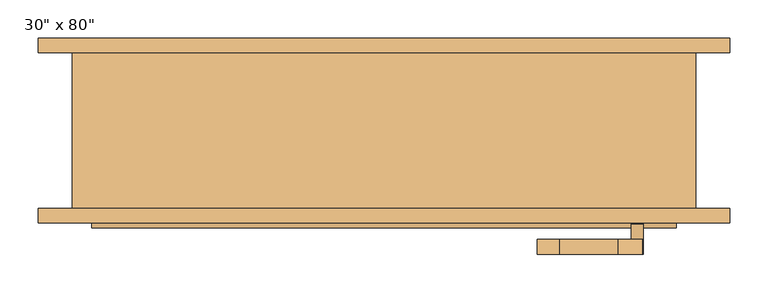
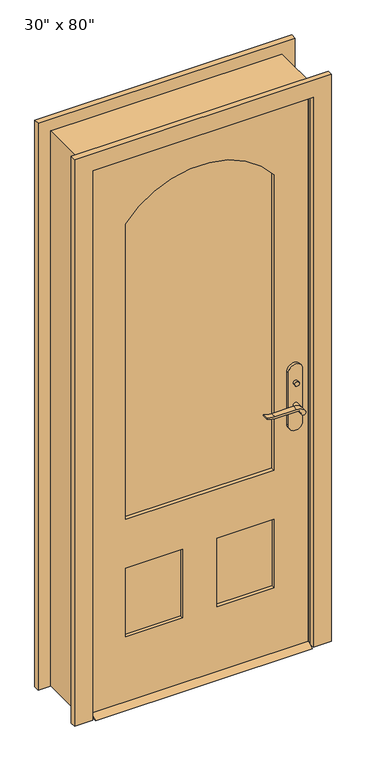
"""IFC4 building model written with IfcOpenShell, lengths in millimetres: door geometry."""

from ifc_helpers import new_model, si_unit, point, frame, frame_2d, origin, place, context, project, spatial, polyline, circle_curve, trimmed, segment, composite_curve, outline, extrude, faceted_brep, source, transform, mapped, element, save


def door_41326d50(model_context):
    return source(origin(), model_context, "Body", "SolidModel", [
        extrude(outline(polyline([(-63.5, 12.7), (-38.1, 0.0), (-123.825, 0.0), (-98.425, 12.7), (-63.5, 12.7)])), frame((-381.0, 0.0, 0.0), z_axis=(1.0, 0.0, 0.0), x_axis=(0.0, 1.0, 0.0)), (0.0, 0.0, 1.0), 762.0),
        extrude(outline(polyline([(335.2, -43.5), (335.2, -53.5), (325.2, -53.5), (325.2, -43.5), (335.2, -43.5)])), frame((0.0, 0.0, 981.9), z_axis=(0.0, 0.0, 1.0), x_axis=(1.0, 0.0, 0.0)), (0.0, 0.0, 1.0), 30.0),
        extrude(outline(composite_curve([segment(trimmed(circle_curve(frame_2d((996.9, 330.2)), 8.0), [point((996.9, 322.2))], [point((996.9, 338.2))], False, "CARTESIAN"), True, "CONTINUOUS"), segment(trimmed(circle_curve(frame_2d((996.9, 330.2)), 8.0), [point((996.9, 338.2))], [point((996.9, 322.2))], False, "CARTESIAN"), True, "CONTINUOUS")], self_intersect=False)), frame((0.0, -118.425, 0.0), z_axis=(0.0, 1.0, 0.0), x_axis=(0.0, 0.0, 1.0)), (0.0, 0.0, 1.0), 10.0),
        extrude(outline(composite_curve([segment(trimmed(circle_curve(frame_2d((897.1555521, 306.5324871)), 37.2832219), [point((919.0523287, 336.7081363))], [point((934.4, 304.8325667))], False, "CARTESIAN"), True, "CONTINUOUS"), segment(polyline([(934.4, 304.8325667), (934.4, 228.5564091)]), True, "CONTINUOUS"), segment(trimmed(circle_curve(frame_2d((1017.6850638, 228.6227909)), 83.2850902), [point((934.4, 228.5564091))], [point((939.4, 200.2))], True, "CARTESIAN"), True, "CONTINUOUS"), segment(polyline([(939.4, 200.2), (936.6135558, 200.2)]), True, "CONTINUOUS"), segment(trimmed(circle_curve(frame_2d((986.6709207, 232.1396612)), 59.3791355), [point((936.6135558, 200.2))], [point((927.4, 228.5564091))], False, "CARTESIAN"), True, "CONTINUOUS"), segment(polyline([(927.4, 228.5564091), (927.4, 304.8138099)]), True, "CONTINUOUS"), segment(trimmed(circle_curve(frame_2d((909.2738613, 304.8138099)), 18.1261387), [point((927.4, 304.8138099))], [point((914.4, 322.2))], True, "CARTESIAN"), True, "CONTINUOUS"), segment(trimmed(circle_curve(frame_2d((914.4, 330.2)), 8.0), [point((914.4, 322.2))], [point((919.0523287, 336.7081363))], False, "CARTESIAN"), True, "CONTINUOUS")], self_intersect=False)), frame((0.0, -23.5, 0.0), z_axis=(0.0, 1.0, 0.0), x_axis=(0.0, 0.0, 1.0)), (0.0, 0.0, 1.0), 20.0),
        extrude(outline(composite_curve([segment(trimmed(circle_curve(frame_2d((914.4, 330.2)), 8.0), [point((914.3999903, 322.2))], [point((919.0523287, 336.7081363))], False, "CARTESIAN"), True, "CONTINUOUS"), segment(trimmed(circle_curve(frame_2d((897.1555521, 306.5324871)), 37.2832219), [point((919.0523287, 336.7081363))], [point((934.4, 304.8325667))], False, "CARTESIAN"), True, "CONTINUOUS"), segment(polyline([(934.4, 304.8325667), (934.4, 228.5564091)]), True, "CONTINUOUS"), segment(trimmed(circle_curve(frame_2d((1017.6850638, 228.6227909)), 83.2850902), [point((934.4, 228.5564091))], [point((939.4, 200.2))], True, "CARTESIAN"), True, "CONTINUOUS"), segment(polyline([(939.4, 200.2), (936.6135558, 200.2)]), True, "CONTINUOUS"), segment(trimmed(circle_curve(frame_2d((986.6709207, 232.1396612)), 59.3791355), [point((936.6135558, 200.2))], [point((927.4, 228.5564091))], False, "CARTESIAN"), True, "CONTINUOUS"), segment(polyline([(927.4, 228.5564091), (927.4, 304.8138122)]), True, "CONTINUOUS"), segment(trimmed(circle_curve(frame_2d((909.2738682, 304.8138122)), 18.1261318), [point((927.4, 304.8138122))], [point((914.3999903, 322.2))], True, "CARTESIAN"), True, "CONTINUOUS")], self_intersect=False)), frame((0.0, -158.425, 0.0), z_axis=(0.0, 1.0, 0.0), x_axis=(0.0, 0.0, 1.0)), (0.0, 0.0, 1.0), 20.0),
        extrude(outline(composite_curve([segment(trimmed(circle_curve(frame_2d((914.4, 330.2)), 8.0), [point((914.4, 322.2))], [point((914.4, 338.2))], False, "CARTESIAN"), True, "CONTINUOUS"), segment(trimmed(circle_curve(frame_2d((914.4, 330.2)), 8.0), [point((914.4, 338.2))], [point((914.4, 322.2))], False, "CARTESIAN"), True, "CONTINUOUS")], self_intersect=False)), frame((0.0, -53.5, 0.0), z_axis=(0.0, 1.0, 0.0), x_axis=(0.0, 0.0, 1.0)), (0.0, 0.0, 1.0), 30.0),
        extrude(outline(composite_curve([segment(trimmed(circle_curve(frame_2d((914.4, 330.2)), 8.0), [point((914.4, 322.2))], [point((914.4, 338.2))], False, "CARTESIAN"), True, "CONTINUOUS"), segment(trimmed(circle_curve(frame_2d((914.4, 330.2)), 8.0), [point((914.4, 338.2))], [point((914.4, 322.2))], False, "CARTESIAN"), True, "CONTINUOUS")], self_intersect=False)), frame((0.0, -138.425, 0.0), z_axis=(0.0, 1.0, 0.0), x_axis=(0.0, 0.0, 1.0)), (0.0, 0.0, 1.0), 30.0),
        extrude(outline(composite_curve([segment(polyline([(844.4, 355.2), (1039.4, 355.2)]), True, "CONTINUOUS"), segment(trimmed(circle_curve(frame_2d((1039.4, 330.2)), 25.0), [point((1039.4, 355.2))], [point((1039.4, 305.2))], False, "CARTESIAN"), True, "CONTINUOUS"), segment(polyline([(1039.4, 305.2), (844.4, 305.2)]), True, "CONTINUOUS"), segment(trimmed(circle_curve(frame_2d((844.4, 330.2)), 25.0), [point((844.4, 305.2))], [point((844.4, 355.2))], False, "CARTESIAN"), True, "CONTINUOUS")], self_intersect=False)), frame((0.0, -63.5, 0.0), z_axis=(0.0, 1.0, 0.0), x_axis=(0.0, 0.0, 1.0)), (0.0, 0.0, 1.0), 10.0),
        extrude(outline(composite_curve([segment(polyline([(844.4, 355.2), (1039.4, 355.2)]), True, "CONTINUOUS"), segment(trimmed(circle_curve(frame_2d((1039.4, 330.2)), 25.0), [point((1039.4, 355.2))], [point((1039.4, 305.2))], False, "CARTESIAN"), True, "CONTINUOUS"), segment(polyline([(1039.4, 305.2), (844.4, 305.2)]), True, "CONTINUOUS"), segment(trimmed(circle_curve(frame_2d((844.4, 330.2)), 25.0), [point((844.4, 305.2))], [point((844.4, 355.2))], False, "CARTESIAN"), True, "CONTINUOUS")], self_intersect=False)), frame((0.0, -108.425, 0.0), z_axis=(0.0, 1.0, 0.0), x_axis=(0.0, 0.0, 1.0)), (0.0, 0.0, 1.0), 10.0),
        extrude(outline(polyline([(2032.0, -381.0), (12.7, -381.0), (12.7, 381.0), (2032.0, 381.0), (2032.0, -381.0)]), holes=[composite_curve([segment(polyline([(688.975, -260.35), (1784.35, -260.35)]), True, "CONTINUOUS"), segment(trimmed(circle_curve(frame_2d((1580.99125, 0.0)), 330.35875), [point((1784.35, -260.35))], [point((1784.35, 260.35))], True, "CARTESIAN"), True, "CONTINUOUS"), segment(polyline([(1784.35, 260.35), (688.975, 260.35), (688.975, -260.35)]), True, "CONTINUOUS")], self_intersect=False), polyline([(508.0, -60.325), (254.0, -60.325), (254.0, -260.35), (508.0, -260.35), (508.0, -60.325)]), polyline([(508.0, 260.35), (254.0, 260.35), (254.0, 60.325), (508.0, 60.325), (508.0, 260.35)])]), frame((0.0, -98.425, 0.0), z_axis=(0.0, 1.0, 0.0), x_axis=(0.0, 0.0, 1.0)), (0.0, 0.0, 1.0), 34.925),
        faceted_brep([(406.4, -98.425, 0.0), (381.0, -98.425, 0.0), (381.0, -63.5, 0.0), (368.3, -63.5, 0.0), (368.3, -28.575, 0.0), (381.0, -28.575, 0.0), (381.0, 104.775, 0.0), (406.4, 104.775, 0.0), (406.4, 104.775, 2057.4), (406.4, -98.425, 2057.4), (381.0, 104.775, 2032.0), (-381.0, 104.775, 2032.0), (-381.0, 104.775, 0.0), (-406.4, 104.775, 0.0), (-406.4, 104.775, 2057.4), (381.0, -28.575, 2032.0), (368.3, -28.575, 2019.3), (-368.3, -28.575, 2019.3), (-368.3, -28.575, 0.0), (-381.0, -28.575, 0.0), (-381.0, -28.575, 2032.0), (368.3, -63.5, 2019.3), (381.0, -63.5, 2032.0), (-381.0, -63.5, 2032.0), (-381.0, -63.5, 0.0), (-368.3, -63.5, 0.0), (-368.3, -63.5, 2019.3), (381.0, -98.425, 2032.0), (-406.4, -98.425, 2057.4), (-406.4, -98.425, 0.0), (-381.0, -98.425, 0.0), (-381.0, -98.425, 2032.0)], [[[0, 1, 2, 3, 4, 5, 6, 7]], [[7, 8, 9, 0]], [[6, 10, 11, 12, 13, 14, 8, 7]], [[5, 15, 10, 6]], [[4, 16, 17, 18, 19, 20, 15, 5]], [[3, 21, 16, 4]], [[2, 22, 23, 24, 25, 26, 21, 3]], [[1, 27, 22, 2]], [[0, 9, 28, 29, 30, 31, 27, 1]], [[8, 14, 28, 9]], [[15, 20, 11, 10]], [[21, 26, 17, 16]], [[27, 31, 23, 22]], [[29, 13, 12, 19, 18, 25, 24, 30]], [[14, 13, 29, 28]], [[20, 19, 12, 11]], [[26, 25, 18, 17]], [[31, 30, 24, 23]]]),
        extrude(outline(polyline([(-60.325, -75.1416667), (-60.325, -86.7833333), (-260.35, -86.7833333), (-260.35, -75.1416667), (-60.325, -75.1416667)])), frame((0.0, 0.0, 254.0), z_axis=(0.0, 0.0, 1.0), x_axis=(1.0, 0.0, 0.0)), (0.0, 0.0, 1.0), 254.0),
        extrude(outline(polyline([(260.35, -75.1416667), (260.35, -86.7833333), (60.325, -86.7833333), (60.325, -75.1416667), (260.35, -75.1416667)])), frame((0.0, 0.0, 254.0), z_axis=(0.0, 0.0, 1.0), x_axis=(1.0, 0.0, 0.0)), (0.0, 0.0, 1.0), 254.0),
        extrude(outline(composite_curve([segment(polyline([(688.975, -260.35), (688.975, 260.35), (1784.35, 260.35)]), True, "CONTINUOUS"), segment(trimmed(circle_curve(frame_2d((1580.99125, 0.0)), 330.35875), [point((1784.35, 260.35))], [point((1784.35, -260.35))], False, "CARTESIAN"), True, "CONTINUOUS"), segment(polyline([(1784.35, -260.35), (688.975, -260.35)]), True, "CONTINUOUS")], self_intersect=False)), frame((0.0, -84.455, 0.0), z_axis=(0.0, 1.0, 0.0), x_axis=(0.0, 0.0, 1.0)), (0.0, 0.0, 1.0), 6.985),
        extrude(outline(polyline([(0.0, -387.35), (2038.35, -387.35), (2038.35, 387.35), (0.0, 387.35), (0.0, 450.85), (2101.85, 450.85), (2101.85, -450.85), (0.0, -450.85), (0.0, -387.35)])), frame((0.0, 104.775, 0.0), z_axis=(0.0, 1.0, 0.0), x_axis=(0.0, 0.0, 1.0)), (0.0, 0.0, 1.0), 19.05),
        extrude(outline(polyline([(0.0, -387.35), (2038.35, -387.35), (2038.35, 387.35), (0.0, 387.35), (0.0, 450.85), (2101.85, 450.85), (2101.85, -450.85), (0.0, -450.85), (0.0, -387.35)])), frame((0.0, -117.475, 0.0), z_axis=(0.0, 1.0, 0.0), x_axis=(0.0, 0.0, 1.0)), (0.0, 0.0, 1.0), 19.05),
    ])


if __name__ == "__main__":
    model = new_model("IFC4")
    model_context = context("Model", 3, world=origin())
    ifc_project = project(units=[si_unit("LENGTHUNIT", "METRE", prefix="MILLI")], contexts=[model_context])
    site = spatial("IfcSite", under=ifc_project)
    building = spatial("IfcBuilding", under=site)
    placement = place(None, origin())
    door_shape = door_41326d50(model_context)
    element("IfcDoor", 1, ObjectType="30\" x 80\"", at=placement, inside=building, context=model_context, shape_type="MappedRepresentation", body=[
        mapped(door_shape, transform((0.0, 0.0, 0.0), x_axis=(1.0, 0.0, 0.0), y_axis=(0.0, 1.0, 0.0), z_axis=(0.0, 0.0, 1.0))),
    ])
    save(model, "model.ifc")

# Revit data of these elements
# Type "30\" x 80\""
#   Type Mark = "9"
#   Assembly Code = "B2030100"
#   Analytic Construction = "French door, wood frame with single glass"
#   Threshold Offset [instance default] = 0' - 0 1/2"
#   Thickness = 0' - 1 3/8"
#   Thermal Resistance (R) = 1.0696 (h·ft²·°F)/BTU
#   Swing Angle [instance default] = 90.00°
#   Stiles = 0' - 4 3/4"
#   Rough Width = 2' - 8"
#   Rough Height = 6' - 9"
#   Radius = 1' - 1.00625"
#   Lock Rail = 0' - 7 1/8"
#   Height = 6' - 8"
#   Width = 2' - 6"
#   Heat Transfer Coefficient (U) = 0.9350 BTU/(h·ft²·°F)
#   Door Offset [instance default] = 0' - 0"
#   Bottom Rail = 0' - 9 1/2"
#   Threshold [instance default] = yes
#   Function = 1
#   Exterior Trim [instance default] = yes
#   Trim Material = Cherry
#   Threshold Material = Cherry
#   Panel Material = Cherry
#   Glazing = Glass
#   Frame Material = Cherry
#   Door Handle Material = Aluminum
#   Visual Light Transmittance = 0
#   Solar Heat Gain Coefficient = 0
#   Wall Closure = (empty or 0)
#   Construction Type = (empty or 0)
# Element 1 (IfcDoor, "30\" x 80\"")
#   Materials on its faces: "Cherry", "Aluminum", "Glass"
# Materials
#   "Cherry": class "Wood", colour RGB 226 177 128, transparency 0, Description = "Prunus Serotina", Cost = 0
#   "Glass": class "Glass", colour RGB 0 128 192, transparency 0.75, Description = "Soda Lime Glass", Cost = 0
#   "Aluminum": class "Metal", colour RGB 247 247 247, transparency 0, Description = "Aluminum 6061", Cost = 0
